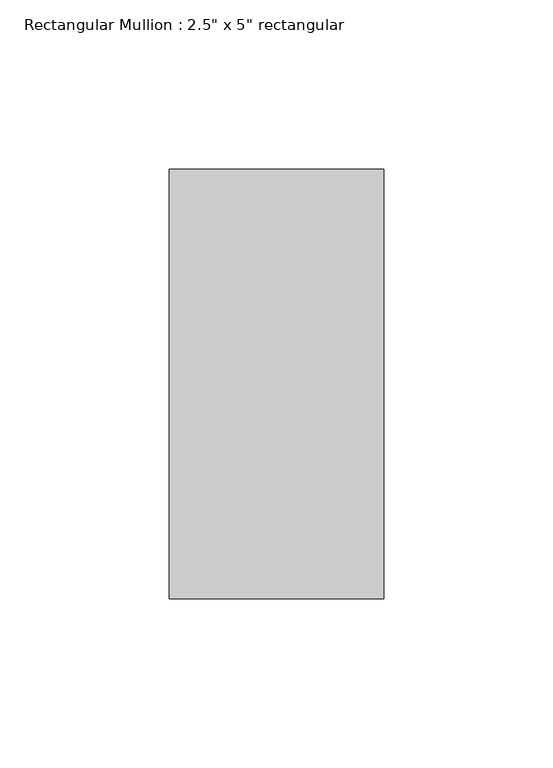
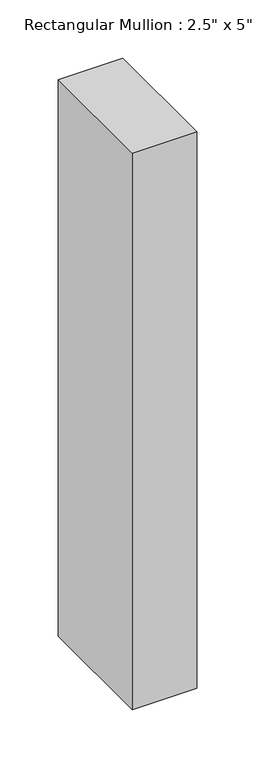
"""IFC4 building model written with IfcOpenShell, lengths in millimetres: member geometry."""

from ifc_helpers import new_model, si_unit, frame, origin, place, context, project, spatial, polyline, outline, extrude, source, transform, mapped, element, save


def member_818e9b4f(model_context):
    return source(origin(), model_context, "Body", "SweptSolid", [
        extrude(outline(polyline([(0.0, 63.5), (0.0, -63.5), (-63.5, -63.5), (-63.5, 63.5), (0.0, 63.5)])), frame((0.0, 0.0, -582.0833333), z_axis=(0.0, 0.0, 1.0), x_axis=(1.0, 0.0, 0.0)), (0.0, 0.0, 1.0), 582.0833333),
    ])


if __name__ == "__main__":
    model = new_model("IFC4")
    model_context = context("Model", 3, world=origin())
    ifc_project = project(units=[si_unit("LENGTHUNIT", "METRE", prefix="MILLI")], contexts=[model_context])
    site = spatial("IfcSite", under=ifc_project)
    building = spatial("IfcBuilding", under=site)
    placement = place(None, origin())
    member_shape = member_818e9b4f(model_context)
    element("IfcMember", 1, ObjectType="Rectangular Mullion : 2.5\" x 5\" rectangular", at=placement, inside=building, context=model_context, shape_type="MappedRepresentation", body=[
        mapped(member_shape, transform((0.0, 0.0, 0.0), x_axis=(1.0, 0.0, 0.0), y_axis=(0.0, 1.0, 0.0), z_axis=(0.0, 0.0, 1.0))),
    ])
    save(model, "model.ifc")

# Revit data of these elements
# Type "Rectangular Mullion : 2.5\" x 5\" rectangular"
#   built-in parameter 1007304 = 0.416667 (stored number, unit not read)
#   built-in parameter 1007301 = 0.104167 (stored number, unit not read)
#   built-in parameter 1007300 = 0.104167 (stored number, unit not read)
# Element 1 (IfcMember, "Rectangular Mullion : 2.5\" x 5\" rectangular")
#   Materials on its faces: "Aluminum"
# Materials
#   "Aluminum": class "Metal", colour RGB 247 247 247, transparency 0, Description = "Aluminum 6061", Cost = 0
